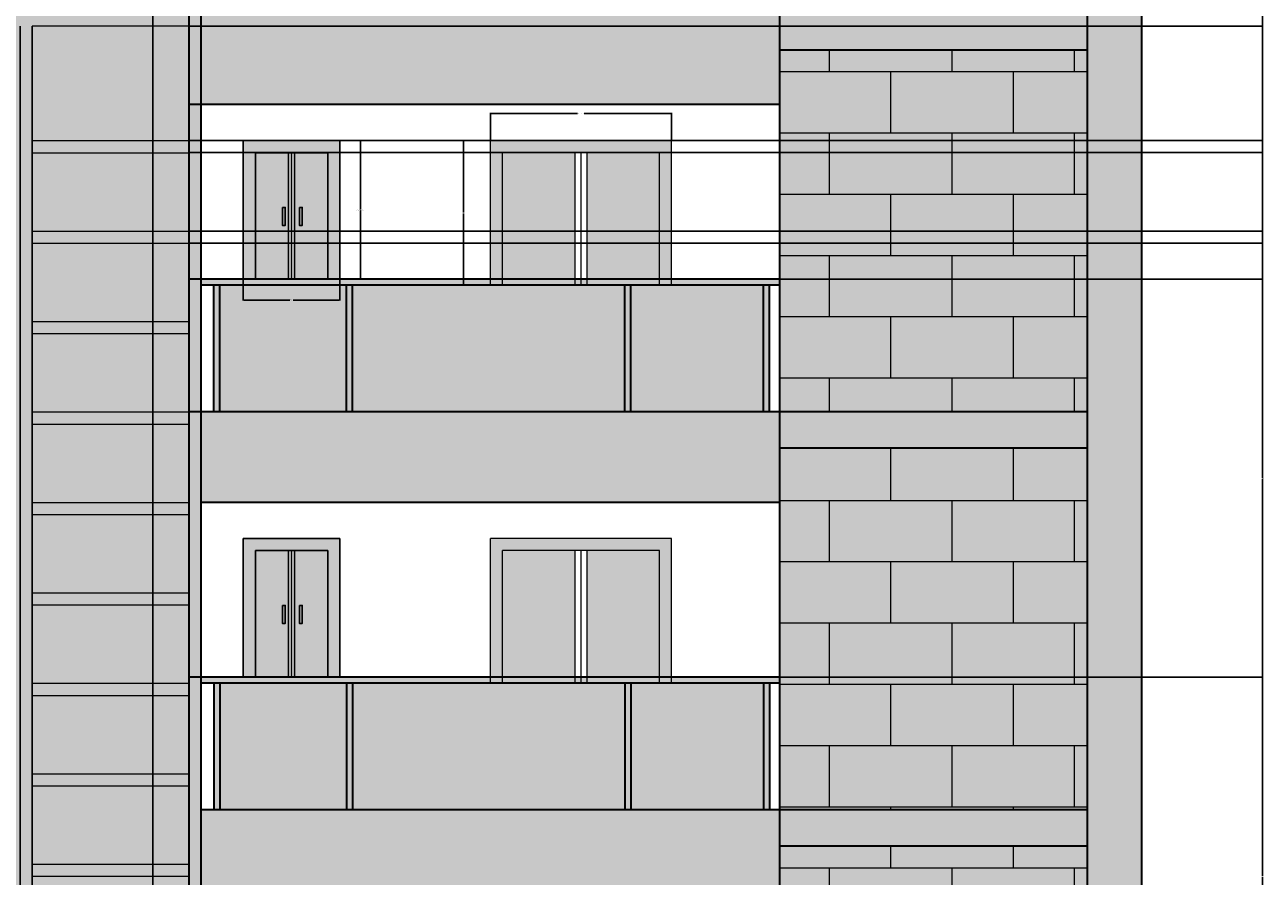
# Model space of a CAD drawing. Units: inches. Extents: x 2794 to 3619, y 522 to 1397.
# Tile 9 of 10: x 3208 to 3619, y 973 to 1255. Entities that reach past the tile are written whole.
import ezdxf

# ---------------------------------------------------------------- set-up
doc = ezdxf.new("R2010")
doc.units = ezdxf.units.IN
for name, color, linetype, lineweight in [('A-ANNO-DIMS', 2, 'Continuous', 18), ('A-DOOR', 3, 'Continuous', 25), ('A-ELEV', 7, 'Continuous', 35), ('A-ELEV-PATT', 8, 'Continuous', 13), ('A-GLAZ', 4, 'Continuous', 18)]:
    doc.layers.add(name, color=color, linetype=linetype, lineweight=lineweight)
doc.styles.get("Standard").update_dxf_attribs({"font": 'arial.ttf'})
doc.dimstyles.get("Standard").update_dxf_attribs({"dimtxt": 0.18, "dimasz": 0.18, "dimexe": 0.18, "dimexo": 0.0625, "dimgap": 0.09, "dimtad": 0, "dimtih": 1, "dimtoh": 1, "dimdec": 4, "dimzin": 0, "dimdsep": 46, "dimtxsty": 'Standard', "dimcen": 0.09, "dimadec": 0, "dimazin": 0, "dimtfac": 1, "dimtdec": 4, "dimtofl": 0, "dimtmove": 0, "dimatfit": 3, "dimfxl": 1, "dimtolj": 1, "dimtzin": 0, "dimarcsym": 0})

# ---------------------------------------------------------------- blocks, each defined once
blk = doc.blocks.new('WIN-1500')
at = {"transparency": 33554646}
h = blk.add_hatch(color=256, dxfattribs=at)
h.dxf.hatch_style = 1
h.paths.add_polyline_path([(60, 48), (0, 48), (0, 2), (4, 2), (4, 44), (56, 44), (56, 2), (60, 2)])
at = {"transparency": 33554687}
h = blk.add_hatch(color=256, dxfattribs=at)
h.dxf.hatch_style = 1
h.set_gradient(color1=(248, 246, 176), color2=(74, 13, 14), name='INVCYLINDER')
h.paths.add_polyline_path([(56, 44), (32, 44), (32, 2), (56, 2)])
h.paths.add_polyline_path([(28, 44), (4, 44), (4, 2), (28, 2)])
for p, q in [((0, 0), (0, 48)), ((60, 48), (0, 48)), ((60, 0), (60, 48)), ((56, 44), (4, 44)), ((4, 0), (4, 44)), ((28, 44), (28, 0)), ((30, 44), (30, 0)), ((32, 44), (32, 0)), ((56, 0), (56, 44))]:
    blk.add_line(p, q)
blk = doc.blocks.new('DOOR-BALCONY-DBL')
at = {"transparency": 33554628}
h = blk.add_hatch(color=256, dxfattribs=at)
h.dxf.hatch_style = 1
h.paths.add_polyline_path([(4, 42), (28, 42), (28, 0), (32, 0), (32, 46), (0, 46), (0, 0), (4, 0)])
at = {"transparency": 33554646}
h = blk.add_hatch(color=256, dxfattribs=at)
h.dxf.hatch_style = 1
h.set_gradient(color1=(255, 255, 255), color2=(147, 149, 152), name='INVCYLINDER')
h.paths.add_polyline_path([(15, 42), (4, 42), (4, 0), (15, 0)])
h = blk.add_hatch(color=256, dxfattribs=at)
h.dxf.hatch_style = 1
h.set_gradient(color1=(255, 255, 255), color2=(147, 149, 152), name='INVCYLINDER')
h.paths.add_polyline_path([(28, 42), (17, 42), (17, 0), (28, 0)])
for p, q in [((0, 0), (0, 46)), ((0, 46), (32, 46)), ((4, 46), (28, 46)), ((32, 0), (32, 46)), ((4, 0), (4, 42)), ((4, 42), (28, 42)), ((15, 0), (15, 42)), ((16, 0), (16, 42)), ((17, 0), (17, 42)), ((28, 0), (28, 42))]:
    blk.add_line(p, q)
for points in [[(12.99, 23.83), (13.93, 23.83), (13.93, 17.87), (12.99, 17.87)], [(18.59, 23.83), (19.53, 23.83), (19.53, 17.87), (18.59, 17.87)]]:
    blk.add_lwpolyline(points, close=True)
blk = doc.blocks.new('*D3')
at = {"layer": 'A-ANNO-DIMS', "color": 0, "lineweight": -2, "transparency": 16777216}
for p, q in [((3362.27, 1216.7), (3362.27, 1225.82)), ((3362.45, 1225.64), (3391.15, 1225.64)), ((3422.09, 1225.64), (3393.38, 1225.64)), ((3422.27, 1216.7), (3422.27, 1225.82))]:
    blk.add_line(p, q, dxfattribs=at)
at = {"layer": 'A-ANNO-DIMS', "color": 0, "transparency": 16777216}
for points in [[(3362.45, 1225.67), (3362.45, 1225.61), (3362.27, 1225.64)], [(3422.09, 1225.67), (3422.09, 1225.61), (3422.27, 1225.64)]]:
    blk.add_solid(points, dxfattribs=at)
at = {"layer": 'Defpoints', "color": 0, "transparency": 16777216}
for p in [(3422.27, 1225.64), (3362.27, 1216.64), (3422.27, 1216.64)]:
    blk.add_point(p, dxfattribs=at)
at = {"layer": 'A-ANNO-DIMS', "color": 0, "transparency": 16777216, "insert": (3392.27, 1225.64), "char_height": 0.18, "attachment_point": 5}
blk.add_mtext('\\A1;WINDOW 60 TYP.', dxfattribs=at)
blk = doc.blocks.new('*D4')
at = {"layer": 'A-ANNO-DIMS', "color": 0, "lineweight": -2, "transparency": 16777216}
for p, q in [((3362.2, 1216.64), (3353.09, 1216.64)), ((3353.27, 1216.46), (3353.27, 1192.82)), ((3353.27, 1168.82), (3353.27, 1192.45)), ((3362.2, 1168.64), (3353.09, 1168.64))]:
    blk.add_line(p, q, dxfattribs=at)
at = {"layer": 'A-ANNO-DIMS', "color": 0, "transparency": 16777216}
for points in [[(3353.24, 1216.46), (3353.3, 1216.46), (3353.27, 1216.64)], [(3353.24, 1168.82), (3353.3, 1168.82), (3353.27, 1168.64)]]:
    blk.add_solid(points, dxfattribs=at)
at = {"layer": 'Defpoints', "color": 0, "transparency": 16777216}
for p in [(3353.27, 1216.64), (3362.27, 1216.64), (3362.27, 1168.64)]:
    blk.add_point(p, dxfattribs=at)
at = {"layer": 'A-ANNO-DIMS', "color": 0, "transparency": 16777216, "insert": (3353.27, 1192.64), "char_height": 0.18, "attachment_point": 5}
blk.add_mtext('\\A1;48 TYP.', dxfattribs=at)
blk = doc.blocks.new('*D5')
at = {"layer": 'A-ANNO-DIMS', "color": 0, "lineweight": -2, "transparency": 16777216}
for p, q in [((3312.33, 1216.64), (3319.35, 1216.64)), ((3319.17, 1216.46), (3319.17, 1193.82)), ((3319.17, 1170.82), (3319.17, 1193.45)), ((3312.33, 1170.64), (3319.35, 1170.64))]:
    blk.add_line(p, q, dxfattribs=at)
at = {"layer": 'A-ANNO-DIMS', "color": 0, "transparency": 16777216}
for points in [[(3319.14, 1216.46), (3319.2, 1216.46), (3319.17, 1216.64)], [(3319.14, 1170.82), (3319.2, 1170.82), (3319.17, 1170.64)]]:
    blk.add_solid(points, dxfattribs=at)
at = {"layer": 'Defpoints', "color": 0, "transparency": 16777216}
for p in [(3312.27, 1216.64), (3319.17, 1216.64), (3312.27, 1170.64)]:
    blk.add_point(p, dxfattribs=at)
at = {"layer": 'A-ANNO-DIMS', "color": 0, "transparency": 16777216, "insert": (3319.17, 1193.64), "char_height": 0.18, "attachment_point": 5}
blk.add_mtext('\\A1;BALCONY DOOR 46 TYP.', dxfattribs=at)
blk = doc.blocks.new('*D6')
at = {"layer": 'A-ANNO-DIMS', "color": 0, "lineweight": -2, "transparency": 16777216}
for p, q in [((3280.27, 1170.57), (3280.27, 1163.56)), ((3312.27, 1170.57), (3312.27, 1163.56)), ((3280.45, 1163.74), (3295.74, 1163.74)), ((3312.09, 1163.74), (3296.79, 1163.74))]:
    blk.add_line(p, q, dxfattribs=at)
at = {"layer": 'A-ANNO-DIMS', "color": 0, "transparency": 16777216}
for points in [[(3280.45, 1163.77), (3280.45, 1163.71), (3280.27, 1163.74)], [(3312.09, 1163.77), (3312.09, 1163.71), (3312.27, 1163.74)]]:
    blk.add_solid(points, dxfattribs=at)
at = {"layer": 'Defpoints', "color": 0, "transparency": 16777216}
for p in [(3280.27, 1170.64), (3312.27, 1170.64), (3312.27, 1163.74)]:
    blk.add_point(p, dxfattribs=at)
at = {"layer": 'A-ANNO-DIMS', "color": 0, "transparency": 16777216, "insert": (3296.27, 1163.74), "char_height": 0.18, "attachment_point": 5}
blk.add_mtext('\\A1;32 TYP.', dxfattribs=at)
blk = doc.blocks.new('*D21')
at = {"layer": 'A-ANNO-DIMS', "color": 0, "lineweight": -2, "transparency": 16777216}
for p, q in [((3458.33, 1038.64), (3618.55, 1038.64)), ((3618.37, 1038.46), (3618.37, 972.82)), ((3618.37, 906.82), (3618.37, 972.45)), ((3458.33, 906.64), (3618.55, 906.64))]:
    blk.add_line(p, q, dxfattribs=at)
at = {"layer": 'A-ANNO-DIMS', "color": 0, "transparency": 16777216}
for points in [[(3618.34, 1038.46), (3618.4, 1038.46), (3618.37, 1038.64)], [(3618.34, 906.82), (3618.4, 906.82), (3618.37, 906.64)]]:
    blk.add_solid(points, dxfattribs=at)
at = {"layer": 'Defpoints', "color": 0, "transparency": 16777216}
for p in [(3458.27, 1038.64), (3618.37, 1038.64), (3458.27, 906.64)]:
    blk.add_point(p, dxfattribs=at)
at = {"layer": 'A-ANNO-DIMS', "color": 0, "transparency": 16777216, "insert": (3618.37, 972.64), "char_height": 0.18, "attachment_point": 5}
blk.add_mtext('\\A1;132', dxfattribs=at)
blk = doc.blocks.new('*D22')
at = {"layer": 'A-ANNO-DIMS', "color": 0, "lineweight": -2, "transparency": 16777216}
for p, q in [((3458.33, 1170.64), (3618.55, 1170.64)), ((3618.37, 1170.46), (3618.37, 1104.82)), ((3618.37, 1038.82), (3618.37, 1104.45)), ((3458.33, 1038.64), (3618.55, 1038.64))]:
    blk.add_line(p, q, dxfattribs=at)
at = {"layer": 'A-ANNO-DIMS', "color": 0, "transparency": 16777216}
for points in [[(3618.34, 1170.46), (3618.4, 1170.46), (3618.37, 1170.64)], [(3618.34, 1038.82), (3618.4, 1038.82), (3618.37, 1038.64)]]:
    blk.add_solid(points, dxfattribs=at)
at = {"layer": 'Defpoints', "color": 0, "transparency": 16777216}
for p in [(3458.27, 1170.64), (3618.37, 1170.64), (3458.27, 1038.64)]:
    blk.add_point(p, dxfattribs=at)
at = {"layer": 'A-ANNO-DIMS', "color": 0, "transparency": 16777216, "insert": (3618.37, 1104.64), "char_height": 0.18, "attachment_point": 5}
blk.add_mtext('\\A1;132', dxfattribs=at)
blk = doc.blocks.new('*D23')
at = {"layer": 'A-ANNO-DIMS', "color": 0, "lineweight": -2, "transparency": 16777216}
for p, q in [((3458.33, 1294.64), (3618.55, 1294.64)), ((3618.37, 1294.46), (3618.37, 1232.82)), ((3618.37, 1170.82), (3618.37, 1232.45)), ((3458.33, 1170.64), (3618.55, 1170.64))]:
    blk.add_line(p, q, dxfattribs=at)
at = {"layer": 'A-ANNO-DIMS', "color": 0, "transparency": 16777216}
for points in [[(3618.34, 1294.46), (3618.4, 1294.46), (3618.37, 1294.64)], [(3618.34, 1170.82), (3618.4, 1170.82), (3618.37, 1170.64)]]:
    blk.add_solid(points, dxfattribs=at)
at = {"layer": 'Defpoints', "color": 0, "transparency": 16777216}
for p in [(3458.27, 1294.64), (3618.37, 1294.64), (3458.27, 1170.64)]:
    blk.add_point(p, dxfattribs=at)
at = {"layer": 'A-ANNO-DIMS', "color": 0, "transparency": 16777216, "insert": (3618.37, 1232.64), "char_height": 0.18, "attachment_point": 5}
blk.add_mtext('\\A1;124', dxfattribs=at)
blk = doc.blocks.new('*D51')
at = {"layer": 'A-ANNO-DIMS', "color": 0, "lineweight": -2, "transparency": 16777216}
for p, q in [((3206.27, 1254.57), (3206.27, 522.36)), ((3210.27, 1254.57), (3210.27, 522.36)), ((3206.45, 522.54), (3208.11, 522.54)), ((3210.09, 522.54), (3208.42, 522.54))]:
    blk.add_line(p, q, dxfattribs=at)
at = {"layer": 'A-ANNO-DIMS', "color": 0, "transparency": 16777216}
for points in [[(3206.45, 522.57), (3206.45, 522.51), (3206.27, 522.54)], [(3210.09, 522.57), (3210.09, 522.51), (3210.27, 522.54)]]:
    blk.add_solid(points, dxfattribs=at)
at = {"layer": 'Defpoints', "color": 0, "transparency": 16777216}
for p in [(3206.27, 1254.64), (3210.27, 1254.64), (3210.27, 522.54)]:
    blk.add_point(p, dxfattribs=at)
at = {"layer": 'A-ANNO-DIMS', "color": 0, "transparency": 16777216, "insert": (3208.27, 522.54), "char_height": 0.18, "attachment_point": 5}
blk.add_mtext('\\A1;4', dxfattribs=at)
blk = doc.blocks.new('*D52')
at = {"layer": 'A-ANNO-DIMS', "color": 0, "lineweight": -2, "transparency": 16777216}
for p, q in [((3210.27, 1254.57), (3210.27, 522.36)), ((3262.27, 1254.57), (3262.27, 522.36)), ((3210.45, 522.54), (3236.05, 522.54)), ((3262.09, 522.54), (3236.48, 522.54))]:
    blk.add_line(p, q, dxfattribs=at)
at = {"layer": 'A-ANNO-DIMS', "color": 0, "transparency": 16777216}
for points in [[(3210.45, 522.57), (3210.45, 522.51), (3210.27, 522.54)], [(3262.09, 522.57), (3262.09, 522.51), (3262.27, 522.54)]]:
    blk.add_solid(points, dxfattribs=at)
at = {"layer": 'Defpoints', "color": 0, "transparency": 16777216}
for p in [(3210.27, 1254.64), (3262.27, 1254.64), (3262.27, 522.54)]:
    blk.add_point(p, dxfattribs=at)
at = {"layer": 'A-ANNO-DIMS', "color": 0, "transparency": 16777216, "insert": (3236.27, 522.54), "char_height": 0.18, "attachment_point": 5}
blk.add_mtext('\\A1;52', dxfattribs=at)
blk = doc.blocks.new('*D53')
at = {"layer": 'A-ANNO-DIMS', "color": 0, "lineweight": -2, "transparency": 16777216}
for p, q in [((3262.33, 1212.64), (3618.55, 1212.64)), ((3618.37, 1212.46), (3618.37, 1199.82)), ((3618.37, 1186.82), (3618.37, 1199.45)), ((3262.33, 1186.64), (3618.55, 1186.64))]:
    blk.add_line(p, q, dxfattribs=at)
at = {"layer": 'A-ANNO-DIMS', "color": 0, "transparency": 16777216}
for points in [[(3618.34, 1212.46), (3618.4, 1212.46), (3618.37, 1212.64)], [(3618.34, 1186.82), (3618.4, 1186.82), (3618.37, 1186.64)]]:
    blk.add_solid(points, dxfattribs=at)
at = {"layer": 'Defpoints', "color": 0, "transparency": 16777216}
for p in [(3262.27, 1212.64), (3618.37, 1212.64), (3262.27, 1186.64)]:
    blk.add_point(p, dxfattribs=at)
at = {"layer": 'A-ANNO-DIMS', "color": 0, "transparency": 16777216, "insert": (3618.37, 1199.64), "char_height": 0.18, "attachment_point": 5}
blk.add_mtext('\\A1;26', dxfattribs=at)
blk = doc.blocks.new('*D54')
at = {"layer": 'A-ANNO-DIMS', "color": 0, "lineweight": -2, "transparency": 16777216}
for p, q in [((3262.328351, 1186.635093), (3618.545851, 1186.635093)), ((3618.365851, 1186.455093), (3618.365851, 1184.815093)), ((3618.365851, 1182.815093), (3618.365851, 1184.455093)), ((3262.328351, 1182.635093), (3618.545851, 1182.635093))]:
    blk.add_line(p, q, dxfattribs=at)
at = {"layer": 'A-ANNO-DIMS', "color": 0, "transparency": 16777216}
for points in [[(3618.335851, 1186.455093), (3618.395851, 1186.455093), (3618.365851, 1186.635093)], [(3618.335851, 1182.815093), (3618.395851, 1182.815093), (3618.365851, 1182.635093)]]:
    blk.add_solid(points, dxfattribs=at)
at = {"layer": 'Defpoints', "color": 0, "transparency": 16777216}
for p in [(3262.265851, 1186.635093), (3618.365851, 1186.635093), (3262.265851, 1182.635093)]:
    blk.add_point(p, dxfattribs=at)
at = {"layer": 'A-ANNO-DIMS', "color": 0, "transparency": 16777216, "insert": (3618.365851, 1184.635093), "char_height": 0.18, "attachment_point": 5}
blk.add_mtext('\\A1;4', dxfattribs=at)
blk = doc.blocks.new('*D55')
at = {"layer": 'A-ANNO-DIMS', "color": 0, "lineweight": -2, "transparency": 16777216}
for p, q in [((3262.33, 1254.64), (3618.55, 1254.64)), ((3618.37, 1254.46), (3618.37, 1235.82)), ((3618.37, 1216.82), (3618.37, 1235.45)), ((3262.33, 1216.64), (3618.55, 1216.64))]:
    blk.add_line(p, q, dxfattribs=at)
at = {"layer": 'A-ANNO-DIMS', "color": 0, "transparency": 16777216}
for points in [[(3618.34, 1254.46), (3618.4, 1254.46), (3618.37, 1254.64)], [(3618.34, 1216.82), (3618.4, 1216.82), (3618.37, 1216.64)]]:
    blk.add_solid(points, dxfattribs=at)
at = {"layer": 'Defpoints', "color": 0, "transparency": 16777216}
for p in [(3262.27, 1254.64), (3618.37, 1254.64), (3262.27, 1216.64)]:
    blk.add_point(p, dxfattribs=at)
at = {"layer": 'A-ANNO-DIMS', "color": 0, "transparency": 16777216, "insert": (3618.37, 1235.64), "char_height": 0.18, "attachment_point": 5}
blk.add_mtext('\\A1;38', dxfattribs=at)
blk = doc.blocks.new('*D56')
at = {"layer": 'A-ANNO-DIMS', "color": 0, "lineweight": -2, "transparency": 16777216}
for p, q in [((3162.27, 664.7), (3162.27, 1396.92)), ((3162.45, 1396.74), (3206.05, 1396.74)), ((3250.09, 1396.74), (3206.49, 1396.74)), ((3250.27, 664.7), (3250.27, 1396.92))]:
    blk.add_line(p, q, dxfattribs=at)
at = {"layer": 'A-ANNO-DIMS', "color": 0, "transparency": 16777216}
for points in [[(3162.45, 1396.77), (3162.45, 1396.71), (3162.27, 1396.74)], [(3250.09, 1396.77), (3250.09, 1396.71), (3250.27, 1396.74)]]:
    blk.add_solid(points, dxfattribs=at)
at = {"layer": 'Defpoints', "color": 0, "transparency": 16777216}
for p in [(3250.27, 1396.74), (3162.27, 664.64), (3250.27, 664.64)]:
    blk.add_point(p, dxfattribs=at)
at = {"layer": 'A-ANNO-DIMS', "color": 0, "transparency": 16777216, "insert": (3206.27, 1396.74), "char_height": 0.18, "attachment_point": 5}
blk.add_mtext('\\A1;88', dxfattribs=at)

msp = doc.modelspace()

# ---------------------------------------------------------------- hatches: boundary and pattern name
at = {"layer": 'A-ELEV-PATT', "transparency": 33554687}
h = msp.add_hatch(color=256, dxfattribs=at)
h.dxf.hatch_style = 1
h.paths.add_polyline_path([(3262.2659, 1350.6351), (3150.2659, 1350.6351), (3150.2659, 1279.0155, -0.68639605), (3262.2659, 1279.0155)])
h.paths.add_polyline_path([(3210.2659, 1314.1121), (3210.2659, 1258.6351), (3262.2659, 1258.6351, 0.39146256)])
h.paths.add_polyline_path([(3206.2659, 1314.2551, 0.41222069), (3150.2659, 1258.6351), (3206.2659, 1258.6351)])
h.paths.add_polyline_path([(3262.2659, 1254.6351), (3210.2659, 1254.6351), (3210.2659, 1216.6351), (3262.2659, 1216.6351)])
h.paths.add_polyline_path([(3206.2659, 1254.6351), (3150.2659, 1254.6351), (3150.2659, 1216.6351), (3206.2659, 1216.6351)])
h.paths.add_polyline_path([(3262.2659, 1212.6351), (3210.2659, 1212.6351), (3210.2659, 1186.6351), (3262.2659, 1186.6351)])
h.paths.add_polyline_path([(3206.2659, 1212.6351), (3150.2659, 1212.6351), (3150.2659, 1186.6351), (3206.2659, 1186.6351)])
h.paths.add_polyline_path([(3206.2659, 1182.6351), (3150.2659, 1182.6351), (3150.2659, 1156.6351), (3206.2659, 1156.6351)])
h.paths.add_polyline_path([(3262.2659, 1182.6351), (3210.2659, 1182.6351), (3210.2659, 1156.6351), (3262.2659, 1156.6351)])
h.paths.add_polyline_path([(3262.2659, 1152.6351), (3210.2659, 1152.6351), (3210.2659, 1126.6351), (3262.2659, 1126.6351)])
h.paths.add_polyline_path([(3206.2659, 1152.6351), (3150.2659, 1152.6351), (3150.2659, 1126.6351), (3206.2659, 1126.6351)])
h.paths.add_polyline_path([(3262.2659, 1122.6351), (3210.2659, 1122.6351), (3210.2659, 1096.6351), (3262.2659, 1096.6351)])
h.paths.add_polyline_path([(3206.2659, 1122.6351), (3150.2659, 1122.6351), (3150.2659, 1096.6351), (3206.2659, 1096.6351)])
h.paths.add_polyline_path([(3206.2659, 1092.6351), (3150.2659, 1092.6351), (3150.2659, 1066.6351), (3206.2659, 1066.6351)])
h.paths.add_polyline_path([(3262.2659, 1092.6351), (3210.2659, 1092.6351), (3210.2659, 1066.6351), (3262.2659, 1066.6351)])
h.paths.add_polyline_path([(3262.2659, 1062.6351), (3210.2659, 1062.6351), (3210.2659, 1036.6351), (3262.2659, 1036.6351)])
h.paths.add_polyline_path([(3206.2659, 1062.6351), (3150.2659, 1062.6351), (3150.2659, 1036.6351), (3206.2659, 1036.6351)])
h.paths.add_polyline_path([(3206.2659, 1032.6351), (3150.2659, 1032.6351), (3150.2659, 1006.6351), (3206.2659, 1006.6351)])
h.paths.add_polyline_path([(3262.2659, 1032.6351), (3210.2659, 1032.6351), (3210.2659, 1006.6351), (3262.2659, 1006.6351)])
h.paths.add_polyline_path([(3262.2659, 1002.6351), (3210.2659, 1002.6351), (3210.2659, 976.6351), (3262.2659, 976.6351)])
h.paths.add_polyline_path([(3206.2659, 1002.6351), (3150.2659, 1002.6351), (3150.2659, 976.6351), (3206.2659, 976.6351)])
h.paths.add_polyline_path([(3206.2659, 972.6351), (3150.2659, 972.6351), (3150.2659, 946.6351), (3206.2659, 946.6351)])
h.paths.add_polyline_path([(3206.2659, 942.6351), (3150.2659, 942.6351), (3150.2659, 916.6351), (3206.2659, 916.6351)])
h.paths.add_polyline_path([(3262.2659, 942.6351), (3210.2659, 942.6351), (3210.2659, 916.6351), (3262.2659, 916.6351)])
h.paths.add_polyline_path([(3262.2659, 972.6351), (3210.2659, 972.6351), (3210.2659, 946.6351), (3262.2659, 946.6351)])
h.paths.add_polyline_path([(3262.2659, 912.6351), (3210.2659, 912.6351), (3210.2659, 886.6351), (3262.2659, 886.6351)])
h.paths.add_polyline_path([(3206.2659, 912.6351), (3150.2659, 912.6351), (3150.2659, 886.6351), (3206.2659, 886.6351)])
h.paths.add_polyline_path([(3206.2659, 882.6351), (3150.2659, 882.6351), (3150.2659, 856.6351), (3206.2659, 856.6351)])
h.paths.add_polyline_path([(3262.2659, 882.6351), (3210.2659, 882.6351), (3210.2659, 856.6351), (3262.2659, 856.6351)])
h.paths.add_polyline_path([(3262.2659, 852.6351), (3210.2659, 852.6351), (3210.2659, 826.6351), (3262.2659, 826.6351)])
h.paths.add_polyline_path([(3206.2659, 852.6351), (3150.2659, 852.6351), (3150.2659, 826.6351), (3206.2659, 826.6351)])
h.paths.add_polyline_path([(3206.2659, 822.6351), (3150.2659, 822.6351), (3150.2659, 796.6351), (3206.2659, 796.6351)])
h.paths.add_polyline_path([(3262.2659, 822.6351), (3210.2659, 822.6351), (3210.2659, 796.6351), (3262.2659, 796.6351)])
h.paths.add_polyline_path([(3262.2659, 792.6351), (3210.2659, 792.6351), (3210.2659, 766.6351), (3262.2659, 766.6351)])
h.paths.add_polyline_path([(3206.2659, 792.6351), (3150.2659, 792.6351), (3150.2659, 766.6351), (3206.2659, 766.6351)])
h.paths.add_polyline_path([(3206.2659, 762.6351), (3150.2659, 762.6351), (3150.2659, 736.6351), (3206.2659, 736.6351)])
h.paths.add_polyline_path([(3206.2659, 732.6351), (3150.2659, 732.6351), (3150.2659, 706.6351), (3206.2659, 706.6351)])
h.paths.add_polyline_path([(3262.2659, 732.6351), (3210.2659, 732.6351), (3210.2659, 706.6351), (3262.2659, 706.6351)])
h.paths.add_polyline_path([(3262.2659, 762.6351), (3210.2659, 762.6351), (3210.2659, 736.6351), (3262.2659, 736.6351)])
h = msp.add_hatch(color=256, dxfattribs=at)
h.dxf.hatch_style = 1
h.paths.add_polyline_path([(3266.2659, 1258.6351, 0.98030963), (3146.2659, 1258.6351), (3150.2659, 1258.6351, -0.9932142), (3262.2659, 1258.6351), (3262.2659, 1228.6351), (3266.2659, 1228.6351)])
h = msp.add_hatch(color=256, dxfattribs=at)
h.dxf.hatch_style = 1
h.paths.add_polyline_path([(3150.2659, 1257.8725, -0.00340445), (3150.2659, 1258.6351), (3146.2659, 1258.6351), (3146.2659, 1228.6351), (3150.2659, 1228.6351)])
h.paths.add_polyline_path([(3262.2659, 1258.6351), (3210.2659, 1258.6351), (3210.2659, 1314.1121, 0.01787385), (3206.2659, 1314.2551), (3206.2659, 1258.6351), (3150.2659, 1258.6351), (3150.2659, 1254.6351), (3206.2659, 1254.6351), (3206.2659, 1216.6351), (3150.2659, 1216.6351), (3150.2659, 1212.6351), (3206.2659, 1212.6351), (3206.2659, 1186.6351), (3150.2659, 1186.6351), (3150.2659, 1182.6351), (3206.2659, 1182.6351), (3206.2659, 1156.6351), (3150.2659, 1156.6351), (3150.2659, 1152.6351), (3206.2659, 1152.6351), (3206.2659, 1126.6351), (3150.2659, 1126.6351), (3150.2659, 1122.6351), (3206.2659, 1122.6351), (3206.2659, 1096.6351), (3150.2659, 1096.6351), (3150.2659, 1092.6351), (3206.2659, 1092.6351), (3206.2659, 1066.6351), (3150.2659, 1066.6351), (3150.2659, 1062.6351), (3206.2659, 1062.6351), (3206.2659, 1036.6351), (3150.2659, 1036.6351), (3150.2659, 1032.6351), (3206.2659, 1032.6351), (3206.2659, 1006.6351), (3150.2659, 1006.6351), (3150.2659, 1002.6351), (3206.2659, 1002.6351), (3206.2659, 976.6351), (3150.2659, 976.6351), (3150.2659, 972.6351), (3206.2659, 972.6351), (3206.2659, 946.6351), (3150.2659, 946.6351), (3150.2659, 942.6351), (3206.2659, 942.6351), (3206.2659, 916.6351), (3150.2659, 916.6351), (3150.2659, 912.6351), (3206.2659, 912.6351), (3206.2659, 886.6351), (3150.2659, 886.6351), (3150.2659, 882.6351), (3206.2659, 882.6351), (3206.2659, 856.6351), (3150.2659, 856.6351), (3150.2659, 852.6351), (3206.2659, 852.6351), (3206.2659, 826.6351), (3150.2659, 826.6351), (3150.2659, 822.6351), (3206.2659, 822.6351), (3206.2659, 796.6351), (3150.2659, 796.6351), (3150.2659, 792.6351), (3206.2659, 792.6351), (3206.2659, 766.6351), (3150.2659, 766.6351), (3150.2659, 762.6351), (3206.2659, 762.6351), (3206.2659, 736.6351), (3150.2659, 736.6351), (3150.2659, 732.6351), (3206.2659, 732.6351), (3206.2659, 706.6351), (3150.2659, 706.6351), (3150.2659, 702.6351), (3262.2659, 702.6351), (3262.2659, 706.6351), (3210.2659, 706.6351), (3210.2659, 732.6351), (3262.2659, 732.6351), (3262.2659, 736.6351), (3210.2659, 736.6351), (3210.2659, 762.6351), (3262.2659, 762.6351), (3262.2659, 766.6351), (3210.2659, 766.6351), (3210.2659, 792.6351), (3262.2659, 792.6351), (3262.2659, 796.6351), (3210.2659, 796.6351), (3210.2659, 822.6351), (3262.2659, 822.6351), (3262.2659, 826.6351), (3210.2659, 826.6351), (3210.2659, 852.6351), (3262.2659, 852.6351), (3262.2659, 856.6351), (3210.2659, 856.6351), (3210.2659, 882.6351), (3262.2659, 882.6351), (3262.2659, 886.6351), (3210.2659, 886.6351), (3210.2659, 912.6351), (3262.2659, 912.6351), (3262.2659, 916.6351), (3210.2659, 916.6351), (3210.2659, 942.6351), (3262.2659, 942.6351), (3262.2659, 946.6351), (3210.2659, 946.6351), (3210.2659, 972.6351), (3262.2659, 972.6351), (3262.2659, 976.6351), (3210.2659, 976.6351), (3210.2659, 1002.6351), (3262.2659, 1002.6351), (3262.2659, 1006.6351), (3210.2659, 1006.6351), (3210.2659, 1032.6351), (3262.2659, 1032.6351), (3262.2659, 1036.6351), (3210.2659, 1036.6351), (3210.2659, 1062.6351), (3262.2659, 1062.6351), (3262.2659, 1066.6351), (3210.2659, 1066.6351), (3210.2659, 1092.6351), (3262.2659, 1092.6351), (3262.2659, 1096.6351), (3210.2659, 1096.6351), (3210.2659, 1122.6351), (3262.2659, 1122.6351), (3262.2659, 1126.6351), (3210.2659, 1126.6351), (3210.2659, 1152.6351), (3262.2659, 1152.6351), (3262.2659, 1156.6351), (3210.2659, 1156.6351), (3210.2659, 1182.6351), (3262.2659, 1182.6351), (3262.2659, 1186.6351), (3210.2659, 1186.6351), (3210.2659, 1212.6351), (3262.2659, 1212.6351), (3262.2659, 1216.6351), (3210.2659, 1216.6351), (3210.2659, 1254.6351), (3262.2659, 1254.6351)])
h = msp.add_hatch(color=256, dxfattribs=at)
h.dxf.hatch_style = 1
h.paths.add_polyline_path([(3578.2659, 1294.6351), (3560.2659, 1294.6351), (3560.2659, 642.6351), (3578.2659, 642.6351)])
h.paths.add_polyline_path([(2852.2659, 1294.6351), (2834.2659, 1294.6351), (2834.2659, 642.6351), (2852.2659, 642.6351)])
h = msp.add_hatch(color=256, dxfattribs=at)
h.dxf.hatch_style = 1
h.paths.add_polyline_path([(2852.2659, 1294.6351), (2834.2659, 1294.6351), (2834.2659, 562.6351), (2852.2659, 562.6351)])
h.paths.add_polyline_path([(3578.2659, 1294.6351), (3560.2659, 1294.6351), (3560.2659, 562.6351), (3578.2659, 562.6351)])
h = msp.add_hatch(color=256, dxfattribs=at)
h.dxf.hatch_style = 1
h.paths.add_polyline_path([(2852.2659, 1246.6351), (2954.2659, 1246.6351), (2954.2659, 1258.6351), (2900.2659, 1258.6351), (2900.2659, 1294.6351), (2852.2659, 1294.6351)])
h.paths.add_polyline_path([(3512.2659, 1294.6351), (3512.2659, 1258.6351), (3458.2659, 1258.6351), (3458.2659, 1246.6351), (3560.2659, 1246.6351), (3560.2659, 1294.6351)])
h.paths.add_polyline_path([(2954.2659, 1114.6351), (2954.2659, 1126.6351), (2852.2659, 1126.6351), (2852.2659, 1114.6351)])
h.paths.add_polyline_path([(3560.2659, 1114.6351), (3560.2659, 1126.6351), (3458.2659, 1126.6351), (3458.2659, 1114.6351)])
h.paths.add_polyline_path([(3560.2659, 982.6351), (3560.2659, 994.6351), (3458.2659, 994.6351), (3458.2659, 982.6351)])
h.paths.add_polyline_path([(2954.2659, 982.6351), (2954.2659, 994.6351), (2852.2659, 994.6351), (2852.2659, 982.6351)])
h.paths.add_polyline_path([(2852.2659, 862.6351), (2852.2659, 850.6351), (2954.2659, 850.6351), (2954.2659, 862.6351)])
h.paths.add_polyline_path([(2852.2659, 730.6351), (2852.2659, 718.6351), (2954.2659, 718.6351), (2954.2659, 730.6351)])
h.paths.add_polyline_path([(3560.2659, 718.6351), (3560.2659, 730.6351), (3458.2659, 730.6351), (3458.2659, 718.6351)])
h.paths.add_polyline_path([(3560.2659, 850.6351), (3560.2659, 862.6351), (3458.2659, 862.6351), (3458.2659, 850.6351)])
h = msp.add_hatch(color=256, dxfattribs=at)
h.dxf.hatch_style = 1
h.paths.add_polyline_path([(3146.2659, 1096.6351), (3146.2659, 1126.6351), (2954.2659, 1126.6351), (2954.2659, 1096.6351)])
h.paths.add_polyline_path([(3458.2659, 1096.6351), (3458.2659, 1126.6351), (3266.2659, 1126.6351), (3266.2659, 1096.6351)])
h.paths.add_polyline_path([(3458.2659, 964.6351), (3458.2659, 994.6351), (3266.2659, 994.6351), (3266.2659, 964.6351)])
h.paths.add_polyline_path([(3146.2659, 964.6351), (3146.2659, 994.6351), (2954.2659, 994.6351), (2954.2659, 964.6351)])
h.paths.add_polyline_path([(3458.2659, 832.6351), (3458.2659, 862.6351), (3266.2659, 862.6351), (3266.2659, 832.6351)])
h.paths.add_polyline_path([(3146.2659, 832.6351), (3146.2659, 862.6351), (2954.2659, 862.6351), (2954.2659, 832.6351)])
h.paths.add_polyline_path([(3458.2659, 700.6351), (3458.2659, 730.6351), (3266.2659, 730.6351), (3266.2659, 700.6351)])
h.paths.add_polyline_path([(3146.2659, 700.6351), (3146.2659, 730.6351), (2954.2659, 730.6351), (2954.2659, 700.6351)])
h.paths.add_polyline_path([(3266.2659, 1294.6351), (3266.2659, 1258.6351), (3266.2659, 1228.6351), (3458.2659, 1228.6351), (3458.2659, 1294.6351)])
h.paths.add_polyline_path([(3146.2659, 1228.6351), (3146.2659, 1256.2485, -0.00994307), (3146.2659, 1258.6351), (3146.2659, 1294.6351), (2954.2659, 1294.6351), (2954.2659, 1228.6351)])
at = {"layer": 'A-ELEV-PATT'}
h = msp.add_hatch(dxfattribs=at)
h.set_pattern_fill('AR-B816', color=256, scale=0.1)
h.paths.add_polyline_path([(2954.2659, 1114.6351), (2852.2659, 1114.6351), (2852.2659, 994.6351), (2954.2659, 994.6351)])
h.paths.add_polyline_path([(2954.2659, 1246.6351), (2852.2659, 1246.6351), (2852.2659, 1126.6351), (2954.2659, 1126.6351)])
h.paths.add_polyline_path([(2954.2659, 982.6351), (2852.2659, 982.6351), (2852.2659, 862.6351), (2954.2659, 862.6351)])
h.paths.add_polyline_path([(2954.2659, 850.6351), (2852.2659, 850.6351), (2852.2659, 730.6351), (2954.2659, 730.6351)])
h.paths.add_polyline_path([(3560.2659, 850.6351), (3458.2659, 850.6351), (3458.2659, 730.6351), (3560.2659, 730.6351)])
h.paths.add_polyline_path([(3560.2659, 982.6351), (3458.2659, 982.6351), (3458.2659, 862.6351), (3560.2659, 862.6351)])
h.paths.add_polyline_path([(3560.2659, 1114.6351), (3458.2659, 1114.6351), (3458.2659, 994.6351), (3560.2659, 994.6351)])
h.paths.add_polyline_path([(3560.2659, 1246.6351), (3458.2659, 1246.6351), (3458.2659, 1126.6351), (3560.2659, 1126.6351)])
h.paths.add_polyline_path([(2852.2659, 642.6351), (2954.2659, 642.6351), (2954.2659, 718.6351), (2852.2659, 718.6351)])
h.paths.add_polyline_path([(3458.2659, 640.6351), (3560.2659, 640.6351), (3560.2659, 718.6351), (3458.2659, 718.6351)])
at = {"layer": 'A-ELEV-PATT', "transparency": 33554630}
h = msp.add_hatch(color=256, dxfattribs=at)
h.dxf.hatch_style = 1
h.paths.add_polyline_path([(2954.2659, 1114.6351), (2852.2659, 1114.6351), (2852.2659, 994.6351), (2954.2659, 994.6351)])
h.paths.add_polyline_path([(2954.2659, 982.6351), (2852.2659, 982.6351), (2852.2659, 862.6351), (2954.2659, 862.6351)])
h.paths.add_polyline_path([(2954.2659, 850.6351), (2852.2659, 850.6351), (2852.2659, 730.6351), (2954.2659, 730.6351)])
h.paths.add_polyline_path([(3560.2659, 850.6351), (3458.2659, 850.6351), (3458.2659, 730.6351), (3560.2659, 730.6351)])
h.paths.add_polyline_path([(3560.2659, 982.6351), (3458.2659, 982.6351), (3458.2659, 862.6351), (3560.2659, 862.6351)])
h.paths.add_polyline_path([(3560.2659, 1114.6351), (3458.2659, 1114.6351), (3458.2659, 994.6351), (3560.2659, 994.6351)])
h.paths.add_polyline_path([(3560.2659, 1246.6351), (3458.2659, 1246.6351), (3458.2659, 1126.6351), (3560.2659, 1126.6351)])
h.paths.add_polyline_path([(2852.2659, 642.6351), (2954.2659, 642.6351), (2954.2659, 718.6351), (2852.2659, 718.6351)])
h.paths.add_polyline_path([(3458.2659, 642.6351), (3560.2659, 642.6351), (3560.2659, 718.6351), (3458.2659, 718.6351)])
at = {"layer": 'A-ELEV-PATT', "transparency": 33554687}
h = msp.add_hatch(color=256, dxfattribs=at)
h.dxf.hatch_style = 1
h.paths.add_polyline_path([(3262.2659, 1170.6351), (3266.2659, 1170.6351), (3266.2659, 1228.6351), (3262.2659, 1228.6351)])
h = msp.add_hatch(color=256, dxfattribs=at)
h.dxf.hatch_style = 1
h.paths.add_polyline_path([(3097.1329, 904.6351), (3095.1329, 904.6351), (3095.1329, 862.6351), (3097.1329, 862.6351)])
h.paths.add_polyline_path([(3143.112, 904.6351), (3141.112, 904.6351), (3141.112, 862.6351), (3143.112, 862.6351)])
h.paths.add_polyline_path([(3146.2659, 906.6351), (2954.2659, 906.6351), (2954.2659, 904.6351), (3146.2659, 904.6351)])
h.paths.add_polyline_path([(3004.8268, 904.6351), (3002.8268, 904.6351), (3002.8268, 862.6351), (3004.8268, 862.6351)])
h.paths.add_polyline_path([(2960.8268, 904.6351), (2958.8268, 904.6351), (2958.8268, 862.6351), (2960.8268, 862.6351)])
h.paths.add_polyline_path([(3146.2659, 1038.6351), (2954.2659, 1038.6351), (2954.2659, 1036.6351), (3146.2659, 1036.6351)])
h.paths.add_polyline_path([(2960.8268, 1036.6351), (2958.8268, 1036.6351), (2958.8268, 994.6351), (2960.8268, 994.6351)])
h.paths.add_polyline_path([(3004.8268, 1036.6351), (3002.8268, 1036.6351), (3002.8268, 994.6351), (3004.8268, 994.6351)])
h.paths.add_polyline_path([(3143.112, 1036.6351), (3141.112, 1036.6351), (3141.112, 994.6351), (3143.112, 994.6351)])
h.paths.add_polyline_path([(3097.1329, 1036.6351), (3095.1329, 1036.6351), (3095.1329, 994.6351), (3097.1329, 994.6351)])
h.paths.add_polyline_path([(3146.2659, 1170.6351), (2954.2659, 1170.6351), (2954.2659, 1168.6351), (3146.2659, 1168.6351)])
h.paths.add_polyline_path([(3004.8268, 1168.6351), (3002.8268, 1168.6351), (3002.8268, 1126.6351), (3004.8268, 1126.6351)])
h.paths.add_polyline_path([(2960.8268, 1168.6351), (2958.8268, 1168.6351), (2958.8268, 1126.6351), (2960.8268, 1126.6351)])
h.paths.add_polyline_path([(3143.112, 1168.6351), (3141.112, 1168.6351), (3141.112, 1126.6351), (3143.112, 1126.6351)])
h.paths.add_polyline_path([(3097.1329, 1168.6351), (3095.1329, 1168.6351), (3095.1329, 1126.6351), (3097.1329, 1126.6351)])
h.paths.add_polyline_path([(3458.2659, 1170.6351), (3266.2659, 1170.6351), (3266.2659, 1168.6351), (3458.2659, 1168.6351)])
h.paths.add_polyline_path([(3272.407, 1168.6351), (3270.407, 1168.6351), (3270.407, 1126.6351), (3272.407, 1126.6351)])
h.paths.add_polyline_path([(3316.407, 1168.6351), (3314.407, 1168.6351), (3314.407, 1126.6351), (3316.407, 1126.6351)])
h.paths.add_polyline_path([(3408.7131, 1168.6351), (3406.7131, 1168.6351), (3406.7131, 1126.6351), (3408.7131, 1126.6351)])
h = msp.add_hatch(color=256, dxfattribs=at)
h.dxf.hatch_style = 1
h.paths.add_polyline_path([(3262.2659, 1126.6351), (3266.2659, 1126.6351), (3266.2659, 1170.6351), (3262.2659, 1170.6351)])
h = msp.add_hatch(color=256, dxfattribs=at)
h.dxf.hatch_style = 1
h.paths.add_polyline_path([(3454.6922, 1168.6351), (3452.6922, 1168.6351), (3452.6922, 1126.6351), (3454.6922, 1126.6351)])
h = msp.add_hatch(color=256, dxfattribs=at)
h.dxf.hatch_style = 1
h.paths.add_polyline_path([(3262.2659, 1038.6351), (3266.2659, 1038.6351), (3266.2659, 1126.6351), (3262.2659, 1126.6351)])
h = msp.add_hatch(color=256, dxfattribs=at)
h.dxf.hatch_style = 1
h.paths.add_polyline_path([(3262.2659, 964.6351), (3266.2659, 964.6351), (3266.2659, 1038.6351), (3262.2659, 1038.6351)])
h = msp.add_hatch(color=256, dxfattribs=at)
h.dxf.hatch_style = 1
h.paths.add_polyline_path([(3458.2659, 1038.6351), (3266.2659, 1038.6351), (3266.2659, 1036.6351), (3458.2659, 1036.6351)])
h.paths.add_polyline_path([(3316.4761, 1036.6351), (3314.4761, 1036.6351), (3314.4761, 994.6351), (3316.4761, 994.6351)])
h.paths.add_polyline_path([(3272.4761, 1036.6351), (3270.4761, 1036.6351), (3270.4761, 994.6351), (3272.4761, 994.6351)])
h.paths.add_polyline_path([(3408.7822, 1036.6351), (3406.7822, 1036.6351), (3406.7822, 994.6351), (3408.7822, 994.6351)])
h.paths.add_polyline_path([(3454.7613, 1036.6351), (3452.7613, 1036.6351), (3452.7613, 994.6351), (3454.7613, 994.6351)])
at = {"layer": 'A-GLAZ', "transparency": 33554556}
h = msp.add_hatch(color=256, dxfattribs=at)
h.dxf.hatch_style = 1
h.set_gradient(color1=(255, 255, 255), color2=(0, 255, 255), name='INVCYLINDER')
h.paths.add_polyline_path([(3314.407, 1168.6351), (3272.407, 1168.6351), (3272.407, 1126.6351), (3314.407, 1126.6351)])
h = msp.add_hatch(color=256, dxfattribs=at)
h.dxf.hatch_style = 1
h.set_gradient(color1=(255, 255, 255), color2=(0, 255, 255), name='INVCYLINDER')
h.paths.add_polyline_path([(3406.7131, 1168.6351), (3316.407, 1168.6351), (3316.407, 1126.6351), (3406.7131, 1126.6351)])
h = msp.add_hatch(color=256, dxfattribs=at)
h.dxf.hatch_style = 1
h.set_gradient(color1=(255, 255, 255), color2=(0, 255, 255), name='INVCYLINDER')
h.paths.add_polyline_path([(3452.6922, 1168.6351), (3408.7131, 1168.6351), (3408.7131, 1126.6351), (3452.6922, 1126.6351)])
h = msp.add_hatch(color=256, dxfattribs=at)
h.dxf.hatch_style = 1
h.set_gradient(color1=(255, 255, 255), color2=(0, 255, 255), name='INVCYLINDER')
h.paths.add_polyline_path([(3314.4761, 1036.6351), (3272.4761, 1036.6351), (3272.4761, 994.6351), (3314.4761, 994.6351)])
h = msp.add_hatch(color=256, dxfattribs=at)
h.dxf.hatch_style = 1
h.set_gradient(color1=(255, 255, 255), color2=(0, 255, 255), name='INVCYLINDER')
h.paths.add_polyline_path([(3406.7822, 1036.6351), (3316.4761, 1036.6351), (3316.4761, 994.6351), (3406.7822, 994.6351)])
h = msp.add_hatch(color=256, dxfattribs=at)
h.dxf.hatch_style = 1
h.set_gradient(color1=(255, 255, 255), color2=(0, 255, 255), name='INVCYLINDER')
h.paths.add_polyline_path([(3452.7613, 1036.6351), (3408.7822, 1036.6351), (3408.7822, 994.6351), (3452.7613, 994.6351)])

# ---------------------------------------------------------------- linework, layer by layer
at = {"layer": 'A-ELEV'}
for p, q in [((3458.2659, 598.6351), (3458.2659, 1294.6351)), ((3560.2659, 562.6351), (3560.2659, 1294.6351)), ((3578.2659, 562.6351), (3578.2659, 1297.6351)), ((3262.2659, 598.6351), (3262.2659, 1258.6351)), ((3266.2659, 598.6351), (3266.2659, 1258.6351)), ((3560.2659, 1246.6351), (3458.2659, 1246.6351)), ((3458.2659, 1228.6351), (3262.2659, 1228.6351)), ((3458.2659, 1170.6351), (3262.2659, 1170.6351)), ((3458.2659, 1168.6351), (3266.2659, 1168.6351)), ((3270.407, 1168.6351), (3270.407, 1126.6351)), ((3272.407, 1168.6351), (3272.407, 1126.6351)), ((3314.407, 1168.6351), (3314.407, 1126.6351)), ((3316.407, 1168.6351), (3316.407, 1126.6351)), ((3406.7131, 1168.6351), (3406.7131, 1126.6351)), ((3408.7131, 1168.6351), (3408.7131, 1126.6351)), ((3452.6922, 1168.6351), (3452.6922, 1126.6351)), ((3454.6922, 1168.6351), (3454.6922, 1126.6351)), ((3560.2659, 1126.6351), (3262.2659, 1126.6351)), ((3560.2659, 1114.6351), (3458.2659, 1114.6351)), ((3458.2659, 1096.6351), (3266.2659, 1096.6351)), ((3458.2659, 1038.6351), (3262.2659, 1038.6351)), ((3458.2659, 1036.6351), (3266.2659, 1036.6351)), ((3270.4761, 1036.6351), (3270.4761, 994.6351)), ((3272.4761, 1036.6351), (3272.4761, 994.6351)), ((3314.4761, 1036.6351), (3314.4761, 994.6351)), ((3316.4761, 1036.6351), (3316.4761, 994.6351)), ((3406.7822, 1036.6351), (3406.7822, 994.6351)), ((3408.7822, 1036.6351), (3408.7822, 994.6351)), ((3452.7613, 1036.6351), (3452.7613, 994.6351)), ((3454.7613, 1036.6351), (3454.7613, 994.6351)), ((3560.2659, 994.6351), (3266.2659, 994.6351)), ((3560.2659, 982.6351), (3458.2659, 982.6351))]:
    msp.add_line(p, q, dxfattribs=at)
at = {"layer": 'A-GLAZ'}
for p, q in [((3262.2659, 1254.6351), (3210.2659, 1254.6351)), ((3210.2659, 1254.6351), (3210.2659, 1216.6351)), ((3210.2659, 1216.6351), (3262.2659, 1216.6351)), ((3210.2659, 1212.6351), (3262.2659, 1212.6351)), ((3210.2659, 1212.6351), (3210.2659, 1186.6351)), ((3210.2659, 1186.6351), (3262.2659, 1186.6351)), ((3210.2659, 1182.6351), (3210.2659, 1156.6351)), ((3210.2659, 1182.6351), (3262.2659, 1182.6351)), ((3210.2659, 1156.6351), (3262.2659, 1156.6351)), ((3210.2659, 1152.6351), (3210.2659, 1126.6351)), ((3210.2659, 1152.6351), (3262.2659, 1152.6351)), ((3210.2659, 1126.6351), (3262.2659, 1126.6351)), ((3210.2659, 1122.6351), (3210.2659, 1096.6351)), ((3210.2659, 1122.6351), (3262.2659, 1122.6351)), ((3210.2659, 1096.6351), (3262.2659, 1096.6351)), ((3210.2659, 1092.6351), (3210.2659, 1066.6351)), ((3210.2659, 1092.6351), (3262.2659, 1092.6351)), ((3210.2659, 1066.6351), (3262.2659, 1066.6351)), ((3210.2659, 1062.6351), (3210.2659, 1036.6351)), ((3210.2659, 1062.6351), (3262.2659, 1062.6351)), ((3210.2659, 1036.6351), (3262.2659, 1036.6351)), ((3210.2659, 1032.6351), (3210.2659, 1006.6351)), ((3210.2659, 1032.6351), (3262.2659, 1032.6351)), ((3210.2659, 1006.6351), (3262.2659, 1006.6351)), ((3210.2659, 1002.6351), (3210.2659, 976.6351)), ((3210.2659, 1002.6351), (3262.2659, 1002.6351)), ((3210.2659, 976.6351), (3262.2659, 976.6351)), ((3210.2659, 972.6351), (3262.2659, 972.6351))]:
    msp.add_line(p, q, dxfattribs=at)

# ---------------------------------------------------------------- block references
at = {"layer": 'A-DOOR'}
for p in [(3280.266, 1170.635), (3280.266, 1038.635)]:
    msp.add_blockref('DOOR-BALCONY-DBL', p, dxfattribs=at)
at = {"layer": 'A-GLAZ'}
for p in [(3362.266, 1168.635), (3362.266, 1036.635)]:
    msp.add_blockref('WIN-1500', p, dxfattribs=at)

# ---------------------------------------------------------------- dimensions: what is measured, and where the dimension line sits
at = {"layer": 'A-ANNO-DIMS'}
for base, p1, p2, picture, middle in [((3250.2659, 1396.7351), (3162.2659, 664.6351), (3250.2659, 664.6351), '*D56', (3206.2659, 1396.7351)), ((3210.2659, 522.5351), (3206.2659, 1254.6351), (3210.2659, 1254.6351), '*D51', (3208.2659, 522.5351)), ((3262.2659, 522.5351), (3210.2659, 1254.6351), (3262.2659, 1254.6351), '*D52', (3236.2659, 522.5351))]:
    dim = msp.add_linear_dim(base=base, p1=p1, p2=p2, dimstyle='Standard', override={"dimdec": 0, "dimlfac": 1, "dimrnd": 0, "dimzin": 0, "dimdsep": 46, "dimlunit": 2}, dxfattribs=at)
    dim.commit()
    dim.dimension.update_dxf_attribs({"geometry": picture, "text_midpoint": middle})
for base, p1, p2, picture, middle in [((3618.3659, 1294.6351), (3458.2659, 1170.6351), (3458.2659, 1294.6351), '*D23', (3618.3659, 1232.6351)), ((3618.3659, 1254.6351), (3262.2659, 1216.6351), (3262.2659, 1254.6351), '*D55', (3618.3659, 1235.6351)), ((3618.3659, 1212.6351), (3262.2659, 1186.6351), (3262.2659, 1212.6351), '*D53', (3618.3659, 1199.6351)), ((3618.3659, 1186.6351), (3262.2659, 1182.6351), (3262.2659, 1186.6351), '*D54', (3618.3659, 1184.6351)), ((3618.3659, 1170.6351), (3458.2659, 1038.6351), (3458.2659, 1170.6351), '*D22', (3618.3659, 1104.6351)), ((3618.3659, 1038.6351), (3458.2659, 906.6351), (3458.2659, 1038.6351), '*D21', (3618.3659, 972.6351))]:
    dim = msp.add_linear_dim(base=base, p1=p1, p2=p2, angle=90, dimstyle='Standard', override={"dimdec": 0, "dimlfac": 1, "dimrnd": 0, "dimzin": 0, "dimdsep": 46, "dimlunit": 2}, dxfattribs=at)
    dim.commit()
    dim.dimension.update_dxf_attribs({"geometry": picture, "text_midpoint": middle})
for base, p1, p2, text, picture, middle in [((3422.2659, 1225.6351), (3362.2659, 1216.6351), (3422.2659, 1216.6351), 'WINDOW <> TYP.', '*D3', (3392.2659, 1225.6351)), ((3312.2659, 1163.7351), (3280.2659, 1170.6351), (3312.2659, 1170.6351), '<> TYP.', '*D6', (3296.2659, 1163.7351))]:
    dim = msp.add_linear_dim(base=base, p1=p1, p2=p2, text=text, dimstyle='Standard', override={"dimdec": 0, "dimrnd": 0, "dimzin": 0, "dimlunit": 2}, dxfattribs=at)
    dim.commit()
    dim.dimension.update_dxf_attribs({"geometry": picture, "text_midpoint": middle})
for base, p1, p2, text, picture, middle in [((3319.1659, 1216.6351), (3312.2659, 1170.6351), (3312.2659, 1216.6351), 'BALCONY DOOR <> TYP.', '*D5', (3319.1659, 1193.6351)), ((3353.2659, 1216.6351), (3362.2659, 1168.6351), (3362.2659, 1216.6351), '<> TYP.', '*D4', (3353.2659, 1192.6351))]:
    dim = msp.add_linear_dim(base=base, p1=p1, p2=p2, angle=90, text=text, dimstyle='Standard', override={"dimdec": 0, "dimrnd": 0, "dimzin": 0, "dimlunit": 2}, dxfattribs=at)
    dim.commit()
    dim.dimension.update_dxf_attribs({"geometry": picture, "text_midpoint": middle})

doc.saveas('drawing.dxf')
